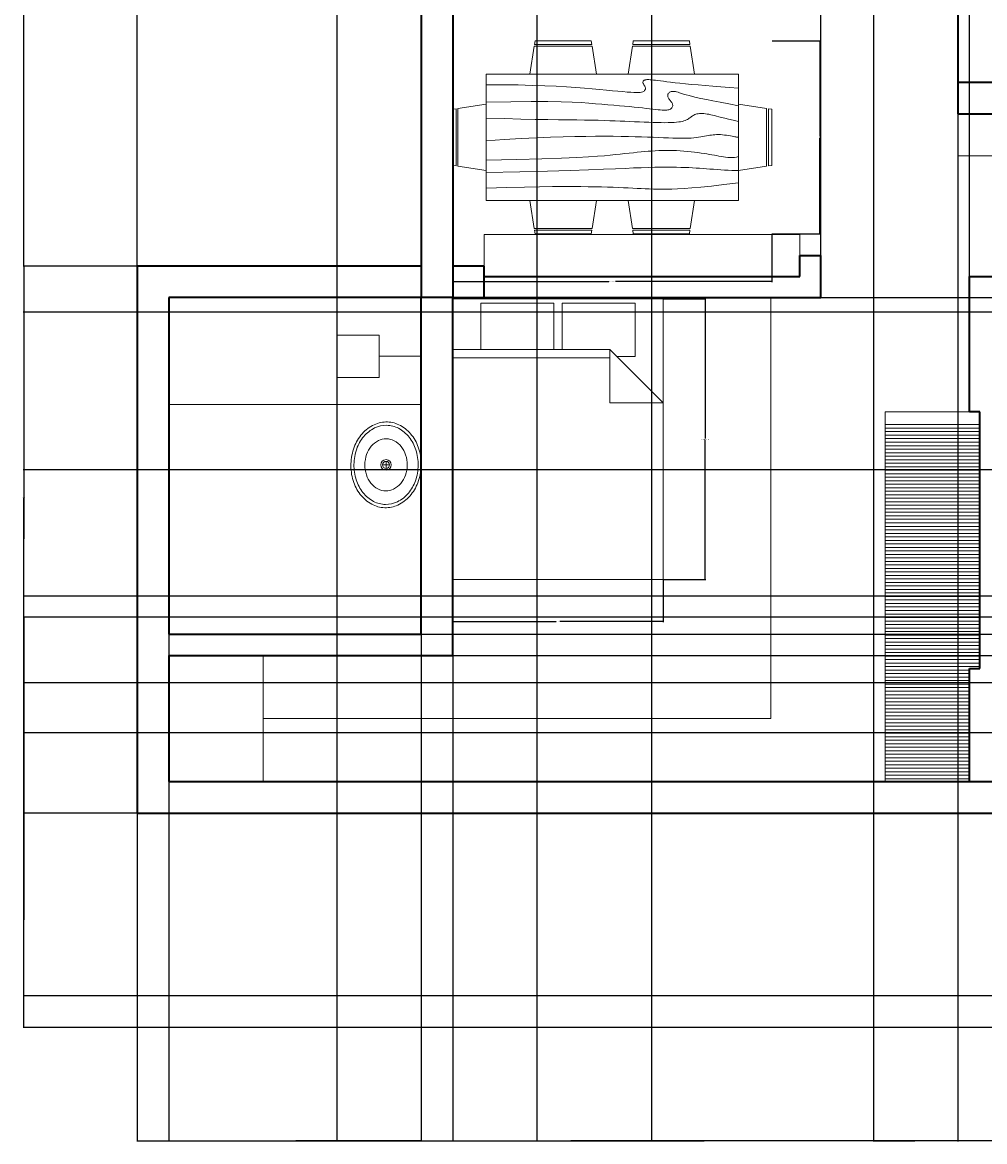
# Model space of a CAD drawing. Units: inches. Extents: x 1159 to 1869, y 2212 to 2738.
# Tile 1 of 5: x 1159 to 1433, y 2212 to 2531. Entities that reach past the tile are written whole.
import ezdxf

# ---------------------------------------------------------------- set-up
doc = ezdxf.new("R2010")
doc.units = ezdxf.units.IN
for name, color, linetype, lineweight in [('A-ANNO-DIMS', 2, 'Continuous', 18), ('A-FLOR', 9, 'Continuous', 13), ('A-FLOR-CASE', 30, 'Continuous', 18), ('A-FLOR-FIXT', 9, 'Continuous', 18), ('A-FLOR-PATT', 252, 'Continuous', 13), ('A-FURN', 8, 'Continuous', 18), ('A-WALL', 7, 'Continuous', 35)]:
    doc.layers.add(name, color=color, linetype=linetype, lineweight=lineweight)
doc.styles.get("Standard").update_dxf_attribs({"font": 'arial.ttf'})
doc.dimstyles.get("Standard").update_dxf_attribs({"dimtxt": 0.18, "dimasz": 0.18, "dimexe": 0.18, "dimexo": 0.0625, "dimgap": 0.09, "dimtad": 0, "dimtih": 1, "dimtoh": 1, "dimdec": 4, "dimzin": 0, "dimdsep": 46, "dimtxsty": 'Standard', "dimcen": 0.09, "dimadec": 0, "dimazin": 0, "dimtfac": 1, "dimtdec": 4, "dimtofl": 0, "dimtmove": 0, "dimatfit": 3, "dimfxl": 1, "dimtolj": 1, "dimtzin": 0, "dimarcsym": 0})

# ---------------------------------------------------------------- blocks, each defined once
blk = doc.blocks.new('Dining Set - 36 x 72 in.')
for p, q in [((-22.2343, 26.00059), (-23.4847, 17.99762)), ((-22.2304, 26), (-5.7608, 26)), ((-22, 27.5), (-22.1562, 26.50042)), ((-5.8416, 26.5), (-22.1534, 26.5)), ((-22, 27.5), (-6, 27.5)), ((-5.8437, 26.49966), (-6, 27.5)), ((-4.5152, 17.99762), (-5.7655, 25.99926)), ((5.7657, 26.00059), (4.5153, 17.99762)), ((5.7696, 26), (22.2392, 26)), ((6, 27.5), (5.8438, 26.50042)), ((22.1584, 26.5), (5.8466, 26.5)), ((6, 27.5), (22, 27.5)), ((22.1563, 26.49966), (22, 27.5)), ((23.4848, 17.99762), (22.2345, 25.99926)), ((36, 18), (-36, 18)), ((-36, 18), (-36, -18)), ((36, -18), (36, 18)), ((-45.5, 8), (-44.5004, 8.15617)), ((-45.5, 8), (-45.5, -8)), ((-44.5, -8.15843), (-44.5, 8.15338)), ((-44.0006, 8.23428), (-35.9976, 9.48474)), ((-44, 8.23041), (-44, -8.23915)), ((44.0006, 8.23428), (35.9976, 9.48474)), ((44, 8.23041), (44, -8.23915)), ((44.5, -8.15843), (44.5, 8.15338)), ((45.5, 8), (44.5005, 8.15617)), ((45.5, 8), (45.5, -8)), ((-44.4997, -8.15631), (-45.5, -8)), ((-35.9976, -9.48476), (-43.9993, -8.2345)), ((35.9976, -9.48476), (43.9993, -8.2345)), ((44.4997, -8.15631), (45.5, -8)), ((-36, -18), (36, -18)), ((-22.2343, -26.0006), (-23.4847, -17.99762)), ((-4.5152, -17.99762), (-5.7655, -25.99928)), ((5.7657, -26.0006), (4.5153, -17.99762)), ((23.4848, -17.99762), (22.2345, -25.99928)), ((-22.2304, -26), (-5.7608, -26)), ((-22, -27.5), (-22.1562, -26.50044)), ((-5.8416, -26.5), (-22.1534, -26.5)), ((-22, -27.5), (-6, -27.5)), ((-5.8437, -26.49967), (-6, -27.5)), ((5.7696, -26), (22.2392, -26)), ((6, -27.5), (5.8438, -26.50044)), ((22.1584, -26.5), (5.8466, -26.5)), ((6, -27.5), (22, -27.5)), ((22.1563, -26.49967), (22, -27.5))]:
    blk.add_line(p, q)
for points in [[(-36, 15), (-31.1772, 14.97754), (-26.8079, 14.91406), (-22.8538, 14.81543), (-19.276, 14.6875), (-16.0362, 14.53613), (-13.0957, 14.36718), (-10.4159, 14.18652), (-7.9583, 14), (-5.6904, 13.81315), (-3.6035, 13.63021), (-1.6954, 13.45508), (0.0365, 13.29166), (1.5945, 13.14388), (2.9811, 13.01562), (4.1988, 12.9108), (5.25, 12.83333), (6.1393, 12.78613), (6.8802, 12.76823), (7.4883, 12.77767), (7.9792, 12.8125), (8.3685, 12.87077), (8.6719, 12.95052), (8.9049, 13.0498), (9.0833, 13.16666), (9.2205, 13.29899), (9.3216, 13.44401), (9.3895, 13.59879), (9.4271, 13.76041), (9.4373, 13.92594), (9.4232, 14.09245), (9.3875, 14.257), (9.3333, 14.41666), (9.2638, 14.56917), (9.1836, 14.71484), (9.0975, 14.85465), (9.0104, 14.98958), (8.9272, 15.1206), (8.8529, 15.2487), (8.7922, 15.37483), (8.75, 15.5), (8.7305, 15.62467), (8.7344, 15.74739), (8.7617, 15.86621), (8.8125, 15.97916), (8.8867, 16.08431), (8.9844, 16.17968), (9.1055, 16.26334), (9.25, 16.33333), (9.4189, 16.38802), (9.6172, 16.42708), (9.8506, 16.45052), (10.125, 16.45833), (10.4463, 16.45052), (10.8203, 16.42708), (11.2529, 16.38802), (11.75, 16.33333), (12.3184, 16.26318), (12.9694, 16.17838), (13.7151, 16.07991), (14.5677, 15.96875), (15.5395, 15.84586), (16.6426, 15.71224), (17.8893, 15.56884), (19.2917, 15.41666), (20.859, 15.25667), (22.5879, 15.08984), (24.4721, 14.91715), (26.5052, 14.73958), (28.6809, 14.5581), (30.9929, 14.3737), (33.4347, 14.18733), (36, 14)], [(-36, 10), (-28.9766, 10.14274), (-23.1725, 10.20442), (-18.4241, 10.19775), (-14.5677, 10.13541), (-11.4399, 10.03011), (-8.877, 9.89453), (-6.7154, 9.74137), (-4.7917, 9.58333), (-2.9698, 9.43082), (-1.2246, 9.28515), (0.4415, 9.14534), (2.026, 9.01041), (3.5266, 8.87939), (4.9408, 8.7513), (6.266, 8.62516), (7.5, 8.5), (8.6411, 8.37549), (9.6914, 8.2539), (10.6538, 8.13818), (11.5312, 8.03125), (12.3267, 7.93603), (13.043, 7.85547), (13.6831, 7.79248), (14.25, 7.75), (14.7471, 7.7303), (15.1797, 7.73307), (15.5537, 7.75732), (15.875, 7.80208), (16.1494, 7.86637), (16.3828, 7.94922), (16.5811, 8.04964), (16.75, 8.16666), (16.8944, 8.29915), (17.0143, 8.44531), (17.1089, 8.60319), (17.1771, 8.77083), (17.218, 8.94629), (17.2305, 9.1276), (17.2137, 9.31282), (17.1667, 9.5), (17.0895, 9.6875), (16.987, 9.875), (16.8649, 10.0625), (16.7292, 10.25), (16.5856, 10.4375), (16.4401, 10.625), (16.2985, 10.8125), (16.1667, 11), (16.05, 11.18733), (15.9518, 11.3737), (15.8752, 11.5581), (15.8229, 11.73958), (15.798, 11.91715), (15.8034, 12.08984), (15.842, 12.25667), (15.9167, 12.41666), (16.0295, 12.56836), (16.1784, 12.70833), (16.3605, 12.83268), (16.5729, 12.9375), (16.8127, 13.01888), (17.0768, 13.07291), (17.3625, 13.0957), (17.6667, 13.08333), (17.9894, 13.03312), (18.3418, 12.94726), (18.7382, 12.82918), (19.1927, 12.68229), (19.7195, 12.51001), (20.3327, 12.31575), (21.0465, 12.10294), (21.875, 11.875), (22.8357, 11.63354), (23.959, 11.37304), (25.2786, 11.08618), (26.8282, 10.76562), (28.6414, 10.40405), (30.752, 9.99414), (33.1936, 9.52856), (36, 9)], [(-36, 5.5), (-30.7157, 5.3348), (-26.069, 5.20963), (-21.9946, 5.11767), (-18.4271, 5.05208), (-15.3009, 5.00602), (-12.5508, 4.97265), (-10.1112, 4.94515), (-7.9167, 4.91666), (-5.909, 4.88167), (-4.0586, 4.83984), (-2.3429, 4.79215), (-0.7396, 4.73958), (0.7739, 4.6831), (2.22, 4.6237), (3.6213, 4.56233), (5, 4.5), (6.373, 4.43782), (7.7344, 4.3776), (9.0723, 4.32129), (10.375, 4.27083), (11.6309, 4.22819), (12.8281, 4.19531), (13.9551, 4.17415), (15, 4.16666), (15.954, 4.17448), (16.819, 4.19791), (17.6001, 4.23698), (18.3021, 4.29166), (18.9299, 4.36198), (19.4883, 4.44791), (19.9823, 4.54948), (20.4167, 4.66666), (20.7969, 4.79899), (21.1302, 4.94401), (21.4245, 5.09879), (21.6875, 5.26041), (21.9271, 5.42594), (22.1511, 5.59245), (22.3672, 5.757), (22.5834, 5.91666), (22.8065, 6.06868), (23.0404, 6.21093), (23.2879, 6.34147), (23.5521, 6.45833), (23.8358, 6.55957), (24.142, 6.64323), (24.4735, 6.70735), (24.8334, 6.75), (25.2235, 6.76969), (25.642, 6.76692), (26.0858, 6.74267), (26.5521, 6.69791), (27.0379, 6.63362), (27.5404, 6.55078), (28.0565, 6.45036), (28.5834, 6.33333), (29.1242, 6.19987), (29.7071, 6.04687), (30.3661, 5.87044), (31.1354, 5.66666), (32.0493, 5.43164), (33.142, 5.16146), (34.4475, 4.85221), (36, 4.5)], [(-36, -1), (-30.7915, -0.6591), (-26.0195, -0.38216), (-21.6519, -0.16284), (-17.6563, 0.00521), (-14.0005, 0.12833), (-10.6523, 0.21289), (-7.5796, 0.26522), (-4.75, 0.29166), (-2.134, 0.29793), (0.2878, 0.28711), (2.5317, 0.26163), (4.6146, 0.22396), (6.5529, 0.17651), (8.3633, 0.12174), (10.0623, 0.06209), (11.6667, 0), (13.1899, -0.06201), (14.6341, -0.1211), (15.9982, -0.17432), (17.2813, -0.21875), (18.4823, -0.25147), (19.6003, -0.26953), (20.6343, -0.27002), (21.5834, -0.25), (22.4481, -0.20768), (23.2357, -0.14584), (23.9549, -0.06836), (24.6146, 0.02083), (25.2235, 0.11784), (25.7904, 0.21875), (26.3241, 0.31966), (26.8334, 0.41666), (27.3265, 0.50618), (27.8099, 0.58593), (28.2894, 0.65397), (28.7709, 0.70833), (29.2601, 0.74707), (29.763, 0.76823), (30.2855, 0.76985), (30.8334, 0.75), (31.4088, 0.70784), (31.9994, 0.64713), (32.589, 0.57275), (33.1615, 0.48958), (33.7008, 0.4025), (34.1908, 0.3164), (34.6153, 0.23616), (34.9584, 0.16666), (35.2099, 0.11165), (35.3848, 0.07031), (35.504, 0.04069), (35.5886, 0.02083), (35.6594, 0.00879), (35.7377, 0.0026), (35.8442, 0.00032), (36, 0)], [(-36, -6.5), (-27.1843, -6.31267), (-20.084, -6.1263), (-14.469, -5.9419), (-10.1094, -5.76042), (-6.7752, -5.58285), (-4.2363, -5.41016), (-2.2629, -5.24333), (-0.625, -5.08334), (0.8708, -4.93099), (2.2715, -4.78646), (3.5872, -4.64974), (4.8281, -4.52084), (6.0046, -4.39974), (7.127, -4.28646), (8.2053, -4.18099), (9.25, -4.08334), (10.2705, -3.99382), (11.2734, -3.91407), (12.2647, -3.84603), (13.25, -3.79167), (14.2354, -3.75293), (15.2266, -3.73177), (16.2295, -3.73015), (17.25, -3.75), (18.2912, -3.79248), (19.3451, -3.85547), (20.4009, -3.93604), (21.4479, -4.03125), (22.4754, -4.13819), (23.4727, -4.25391), (24.4289, -4.37549), (25.3334, -4.5), (26.1785, -4.62492), (26.9694, -4.74935), (27.7145, -4.87281), (28.4219, -4.99479), (29.1, -5.11483), (29.7572, -5.23242), (30.4016, -5.34709), (31.0417, -5.45834), (31.6837, -5.56437), (32.3262, -5.65821), (32.9658, -5.73153), (33.599, -5.77604), (34.2224, -5.78345), (34.8327, -5.74545), (35.4264, -5.65373), (36, -5.5)], [(-36, -10), (-26.4022, -9.81299), (-18.4675, -9.62891), (-11.9839, -9.45069), (-6.7396, -9.28125), (-2.5226, -9.12354), (0.8789, -8.98047), (3.6769, -8.85498), (6.0833, -8.75), (8.2767, -8.66765), (10.3021, -8.60677), (12.1712, -8.56543), (13.8958, -8.54167), (15.4876, -8.53353), (16.9583, -8.53907), (18.3197, -8.55632), (19.5834, -8.58334), (20.7616, -8.61841), (21.8685, -8.66081), (22.9188, -8.71004), (23.9271, -8.76563), (24.9081, -8.82707), (25.8763, -8.89388), (26.8465, -8.96558), (27.8334, -9.04167), (28.8474, -9.12118), (29.8828, -9.20117), (30.93, -9.27824), (31.9792, -9.34896), (33.0205, -9.40991), (34.0443, -9.45768), (35.0407, -9.48885), (36, -9.5)], [(-36, -14.5), (-30.0881, -14.33513), (-25.0332, -14.21224), (-20.7312, -14.12647), (-17.0781, -14.07292), (-13.97, -14.04671), (-11.3027, -14.04297), (-8.9724, -14.05681), (-6.875, -14.08334), (-4.9224, -14.11833), (-3.0905, -14.16016), (-1.3709, -14.20785), (0.2448, -14.26042), (1.7647, -14.3169), (3.1973, -14.3763), (4.5507, -14.43767), (5.8333, -14.5), (7.0554, -14.5621), (8.235, -14.62175), (9.3922, -14.67652), (10.5469, -14.72396), (11.7192, -14.76164), (12.929, -14.78711), (14.1965, -14.79794), (15.5417, -14.79167), (16.9933, -14.76424), (18.6152, -14.70508), (20.4804, -14.60197), (22.6615, -14.44271), (25.2312, -14.21509), (28.2624, -13.9069), (31.8277, -13.50594), (36, -13)]]:
    blk.add_lwpolyline(points)
blk = doc.blocks.new('Bed - Queen')
for p, q in [((0, -80.00003), (0, 0)), ((0, 0), (59.99999, 0)), ((59.99999, 0), (59.99999, -80.00003)), ((7.99999, -1.2), (28.79998, -1.2)), ((7.99999, -14.4), (7.99999, -1.2)), ((28.79998, -1.2), (28.79998, -14.4)), ((31.19999, -1.2), (51.99999, -1.2)), ((31.19999, -14.4), (31.19999, -1.2)), ((51.99999, -1.2), (51.99999, -16.4)), ((0, -14.4), (44.8, -14.4)), ((59.99999, -29.6), (44.8, -14.4)), ((44.8, -14.4), (44.8, -29.6)), ((44.8, -16.8), (0, -16.8)), ((51.99999, -16.4), (46.79936, -16.4)), ((44.8, -29.6), (59.99999, -29.6)), ((59.99999, -80.00003), (0, -80.00003))]:
    blk.add_line(p, q)
blk = doc.blocks.new('Sink - Oval top')
for p, q in [((-1, 0), (1, 0)), ((0, 1), (0, -1))]:
    blk.add_line(p, q)
for points in [[(-12.23, 0.39, 0.117634), (-11.46, -3.36, 0.104469), (-8.88, -6.8, 0.090016), (-5.08, -9.07, 0.08192), (-0.32, -10.02, 0.08192), (4.49, -9.38, 0.090016), (8.42, -7.36, 0.104469), (11.22, -4.09, 0.117634), (12.23, -0.39, 0.117634), (11.46, 3.36, 0.104469), (8.88, 6.8, 0.090016), (5.08, 9.07, 0.08192), (0.32, 10.02, 0.08192), (-4.49, 9.38, 0.090016), (-8.42, 7.36, 0.104469), (-11.22, 4.09, 0.117634)], [(-11.29, 0.16, 0.118622), (-10.52, -3.25, 0.104678), (-8.07, -6.36, 0.089562), (-4.54, -8.37, 0.081185), (-0.13, -9.15, 0.081185), (4.3, -8.49, 0.089562), (7.89, -6.58, 0.104678), (10.42, -3.55, 0.118622), (11.29, -0.16, 0.118622), (10.52, 3.25, 0.104678), (8.07, 6.36, 0.089562), (4.54, 8.37, 0.081185), (0.13, 9.15, 0.081185), (-4.3, 8.49, 0.089562), (-7.89, 6.58, 0.104678), (-10.42, 3.55, 0.118622)], [(-7.42, 0.08, 0.118283), (-6.91, -2.17, 0.104607), (-5.29, -4.21, 0.089718), (-2.97, -5.53, 0.081436), (-0.07, -6.04, 0.081436), (2.84, -5.59, 0.089718), (5.2, -4.33, 0.104607), (6.86, -2.32, 0.118283), (7.42, -0.08, 0.118283), (6.91, 2.17, 0.104607), (5.29, 4.21, 0.089718), (2.97, 5.53, 0.081436), (0.07, 6.04, 0.081436), (-2.84, 5.59, 0.089718), (-5.2, 4.33, 0.104607), (-6.86, 2.32, 0.118283)]]:
    blk.add_lwpolyline(points, format="xyb", close=True)
for radius in [1.5, 1]:
    blk.add_circle((0, 0), radius)
blk = doc.blocks.new('SHOWER-HEAD-SQUARE-12IN')
for p, q in [((6, 12), (0, 12)), ((0, 12), (0, 0)), ((12, 12), (6, 12)), ((12, 0), (12, 12)), ((0, 0), (12, 0))]:
    blk.add_line(p, q)
blk = doc.blocks.new('*D10')
at = {"layer": 'A-ANNO-DIMS', "color": 0, "lineweight": -2, "transparency": 16777216}
for p, q in [((1341.46, 2451.83), (1353.58, 2451.83)), ((1353.4, 2451.65), (1353.4, 2412.02)), ((1353.4, 2372.01), (1353.4, 2411.65)), ((1341.46, 2371.83), (1353.58, 2371.83))]:
    blk.add_line(p, q, dxfattribs=at)
at = {"layer": 'A-ANNO-DIMS', "color": 0, "transparency": 16777216}
for points in [[(1353.37, 2451.65), (1353.43, 2451.65), (1353.4, 2451.83)], [(1353.37, 2372.01), (1353.43, 2372.01), (1353.4, 2371.83)]]:
    blk.add_solid(points, dxfattribs=at)
at = {"layer": 'Defpoints', "color": 0, "transparency": 16777216}
for p in [(1341.4, 2451.83), (1353.4, 2451.83), (1341.4, 2371.83)]:
    blk.add_point(p, dxfattribs=at)
at = {"layer": 'A-ANNO-DIMS', "color": 0, "transparency": 16777216, "insert": (1353.4, 2411.83), "char_height": 0.18, "attachment_point": 5}
blk.add_mtext('\\A1;QUEEN BED 80 TYP.', dxfattribs=at)
blk = doc.blocks.new('*D11')
at = {"layer": 'A-ANNO-DIMS', "color": 0, "lineweight": -2, "transparency": 16777216}
for p, q in [((1281.4, 2371.77), (1281.4, 2359.65)), ((1341.4, 2371.77), (1341.4, 2359.65)), ((1281.58, 2359.83), (1310.87, 2359.83)), ((1341.22, 2359.83), (1311.93, 2359.83))]:
    blk.add_line(p, q, dxfattribs=at)
at = {"layer": 'A-ANNO-DIMS', "color": 0, "transparency": 16777216}
for points in [[(1281.58, 2359.86), (1281.58, 2359.8), (1281.4, 2359.83)], [(1341.22, 2359.86), (1341.22, 2359.8), (1341.4, 2359.83)]]:
    blk.add_solid(points, dxfattribs=at)
at = {"layer": 'Defpoints', "color": 0, "transparency": 16777216}
for p in [(1281.4, 2371.83), (1341.4, 2371.83), (1341.4, 2359.83)]:
    blk.add_point(p, dxfattribs=at)
at = {"layer": 'A-ANNO-DIMS', "color": 0, "transparency": 16777216, "insert": (1311.4, 2359.83), "char_height": 0.18, "attachment_point": 5}
blk.add_mtext('\\A1;60 TYP.', dxfattribs=at)
blk = doc.blocks.new('*D14')
at = {"layer": 'A-ANNO-DIMS', "color": 0, "lineweight": -2, "transparency": 16777216}
for p, q in [((1281.4, 2470.37), (1281.4, 2456.61)), ((1372.4, 2470.37), (1372.4, 2456.61)), ((1281.58, 2456.79), (1325.95, 2456.79)), ((1372.22, 2456.79), (1327.85, 2456.79))]:
    blk.add_line(p, q, dxfattribs=at)
at = {"layer": 'A-ANNO-DIMS', "color": 0, "transparency": 16777216}
for points in [[(1281.58, 2456.82), (1281.58, 2456.76), (1281.4, 2456.79)], [(1372.22, 2456.82), (1372.22, 2456.76), (1372.4, 2456.79)]]:
    blk.add_solid(points, dxfattribs=at)
at = {"layer": 'Defpoints', "color": 0, "transparency": 16777216}
for p in [(1281.4, 2470.44), (1372.4, 2470.44), (1372.4, 2456.79)]:
    blk.add_point(p, dxfattribs=at)
at = {"layer": 'A-ANNO-DIMS', "color": 0, "transparency": 16777216, "insert": (1326.9, 2456.79), "char_height": 0.18, "attachment_point": 5}
blk.add_mtext('\\A1;DINING SET 91', dxfattribs=at)
blk = doc.blocks.new('*D15')
at = {"layer": 'A-ANNO-DIMS', "color": 0, "lineweight": -2, "transparency": 16777216}
for p, q in [((1372.46, 2525.44), (1386.23, 2525.44)), ((1386.05, 2525.26), (1386.05, 2498.12)), ((1386.05, 2470.62), (1386.05, 2497.75)), ((1372.46, 2470.44), (1386.23, 2470.44))]:
    blk.add_line(p, q, dxfattribs=at)
at = {"layer": 'A-ANNO-DIMS', "color": 0, "transparency": 16777216}
for points in [[(1386.02, 2525.26), (1386.08, 2525.26), (1386.05, 2525.44)], [(1386.02, 2470.62), (1386.08, 2470.62), (1386.05, 2470.44)]]:
    blk.add_solid(points, dxfattribs=at)
at = {"layer": 'Defpoints', "color": 0, "transparency": 16777216}
for p in [(1372.4, 2525.44), (1386.05, 2525.44), (1372.4, 2470.44)]:
    blk.add_point(p, dxfattribs=at)
at = {"layer": 'A-ANNO-DIMS', "color": 0, "transparency": 16777216, "insert": (1386.05, 2497.94), "char_height": 0.18, "attachment_point": 5}
blk.add_mtext('\\A1;55', dxfattribs=at)
blk = doc.blocks.new('*D20')
at = {"layer": 'A-ANNO-DIMS', "color": 0, "lineweight": -2, "transparency": 16777216}
for p, q in [((1191.4, 2461.27), (1191.4, 2738.15)), ((1191.58, 2737.97), (1513.61, 2737.97)), ((1836.22, 2737.97), (1514.19, 2737.97)), ((1836.4, 2705.69), (1836.4, 2738.15))]:
    blk.add_line(p, q, dxfattribs=at)
at = {"layer": 'A-ANNO-DIMS', "color": 0, "transparency": 16777216}
for points in [[(1191.58, 2738), (1191.58, 2737.94), (1191.4, 2737.97)], [(1836.22, 2738), (1836.22, 2737.94), (1836.4, 2737.97)]]:
    blk.add_solid(points, dxfattribs=at)
at = {"layer": 'Defpoints', "color": 0, "transparency": 16777216}
for p in [(1836.4, 2737.97), (1836.4, 2705.63), (1191.4, 2461.21)]:
    blk.add_point(p, dxfattribs=at)
at = {"layer": 'A-ANNO-DIMS', "color": 0, "transparency": 16777216, "insert": (1513.9, 2737.97), "char_height": 0.18, "attachment_point": 5}
blk.add_mtext('\\A1;645', dxfattribs=at)
blk = doc.blocks.new('*D22')
at = {"layer": 'A-ANNO-DIMS', "color": 0, "lineweight": -2, "transparency": 16777216}
for p, q in [((1191.4, 2461.27), (1191.4, 2738.15)), ((1191.58, 2737.97), (1231.7, 2737.97)), ((1272.22, 2737.97), (1232.1, 2737.97)), ((1272.4, 2461.27), (1272.4, 2738.15))]:
    blk.add_line(p, q, dxfattribs=at)
at = {"layer": 'A-ANNO-DIMS', "color": 0, "transparency": 16777216}
for points in [[(1191.58, 2738), (1191.58, 2737.94), (1191.4, 2737.97)], [(1272.22, 2738), (1272.22, 2737.94), (1272.4, 2737.97)]]:
    blk.add_solid(points, dxfattribs=at)
at = {"layer": 'Defpoints', "color": 0, "transparency": 16777216}
for p in [(1272.4, 2737.97), (1191.4, 2461.21), (1272.4, 2461.21)]:
    blk.add_point(p, dxfattribs=at)
at = {"layer": 'A-ANNO-DIMS', "color": 0, "transparency": 16777216, "insert": (1231.9, 2737.97), "char_height": 0.18, "attachment_point": 5}
blk.add_mtext('\\A1;81', dxfattribs=at)
blk = doc.blocks.new('*D23')
at = {"layer": 'A-ANNO-DIMS', "color": 0, "lineweight": -2, "transparency": 16777216}
for p, q in [((1425.4, 2556.85), (1425.4, 2211.56)), ((1281.4, 2548.45), (1281.4, 2211.56)), ((1281.58, 2211.74), (1353.12, 2211.74)), ((1425.22, 2211.74), (1353.68, 2211.74))]:
    blk.add_line(p, q, dxfattribs=at)
at = {"layer": 'A-ANNO-DIMS', "color": 0, "transparency": 16777216}
for points in [[(1281.58, 2211.77), (1281.58, 2211.71), (1281.4, 2211.74)], [(1425.22, 2211.77), (1425.22, 2211.71), (1425.4, 2211.74)]]:
    blk.add_solid(points, dxfattribs=at)
at = {"layer": 'Defpoints', "color": 0, "transparency": 16777216}
for p in [(1425.4, 2556.91), (1281.4, 2548.52), (1425.4, 2211.74)]:
    blk.add_point(p, dxfattribs=at)
at = {"layer": 'A-ANNO-DIMS', "color": 0, "transparency": 16777216, "insert": (1353.4, 2211.74), "char_height": 0.18, "attachment_point": 5}
blk.add_mtext('\\A1;144', dxfattribs=at)
blk = doc.blocks.new('*D26')
at = {"layer": 'A-ANNO-DIMS', "color": 0, "lineweight": -2, "transparency": 16777216}
for p, q in [((1191.4, 2305.14), (1191.4, 2211.56)), ((1437.74, 2305.14), (1437.74, 2211.56)), ((1191.58, 2211.74), (1314.11, 2211.74)), ((1437.56, 2211.74), (1315.04, 2211.74))]:
    blk.add_line(p, q, dxfattribs=at)
at = {"layer": 'A-ANNO-DIMS', "color": 0, "transparency": 16777216}
for points in [[(1191.58, 2211.77), (1191.58, 2211.71), (1191.4, 2211.74)], [(1437.56, 2211.77), (1437.56, 2211.71), (1437.74, 2211.74)]]:
    blk.add_solid(points, dxfattribs=at)
at = {"layer": 'Defpoints', "color": 0, "transparency": 16777216}
for p in [(1191.4, 2305.21), (1437.74, 2305.21), (1437.74, 2211.74)]:
    blk.add_point(p, dxfattribs=at)
at = {"layer": 'A-ANNO-DIMS', "color": 0, "transparency": 16777216, "insert": (1314.57, 2211.74), "char_height": 0.18, "attachment_point": 5}
blk.add_mtext('\\A1;246.34', dxfattribs=at)
blk = doc.blocks.new('*D29')
at = {"layer": 'A-ANNO-DIMS', "color": 0, "lineweight": -2, "transparency": 16777216}
for p, q in [((1191.34, 2461.21), (1158.88, 2461.21)), ((1159.06, 2461.03), (1159.06, 2383.39)), ((1159.06, 2305.39), (1159.06, 2383.02)), ((1191.34, 2305.21), (1158.88, 2305.21))]:
    blk.add_line(p, q, dxfattribs=at)
at = {"layer": 'A-ANNO-DIMS', "color": 0, "transparency": 16777216}
for points in [[(1159.03, 2461.03), (1159.09, 2461.03), (1159.06, 2461.21)], [(1159.03, 2305.39), (1159.09, 2305.39), (1159.06, 2305.21)]]:
    blk.add_solid(points, dxfattribs=at)
at = {"layer": 'Defpoints', "color": 0, "transparency": 16777216}
for p in [(1159.06, 2461.21), (1191.4, 2461.21), (1191.4, 2305.21)]:
    blk.add_point(p, dxfattribs=at)
at = {"layer": 'A-ANNO-DIMS', "color": 0, "transparency": 16777216, "insert": (1159.06, 2383.21), "char_height": 0.18, "attachment_point": 5}
blk.add_mtext('\\A1;156', dxfattribs=at)
blk = doc.blocks.new('*D30')
at = {"layer": 'A-ANNO-DIMS', "color": 0, "lineweight": -2, "transparency": 16777216}
for p, q in [((1272.34, 2705.63), (1158.88, 2705.63)), ((1159.06, 2705.45), (1159.06, 2583.6)), ((1159.06, 2461.39), (1159.06, 2583.24)), ((1191.34, 2461.21), (1158.88, 2461.21))]:
    blk.add_line(p, q, dxfattribs=at)
at = {"layer": 'A-ANNO-DIMS', "color": 0, "transparency": 16777216}
for points in [[(1159.03, 2705.45), (1159.09, 2705.45), (1159.06, 2705.63)], [(1159.03, 2461.39), (1159.09, 2461.39), (1159.06, 2461.21)]]:
    blk.add_solid(points, dxfattribs=at)
at = {"layer": 'Defpoints', "color": 0, "transparency": 16777216}
for p in [(1159.06, 2705.63), (1272.4, 2705.63), (1191.4, 2461.21)]:
    blk.add_point(p, dxfattribs=at)
at = {"layer": 'A-ANNO-DIMS', "color": 0, "transparency": 16777216, "insert": (1159.06, 2583.42), "char_height": 0.18, "attachment_point": 5}
blk.add_mtext('\\A1;244.4', dxfattribs=at)
blk = doc.blocks.new('*D41')
at = {"layer": 'A-ANNO-DIMS', "color": 0, "lineweight": -2, "transparency": 16777216}
for p, q in [((1200.4, 2356.14), (1200.4, 2211.56)), ((1272.4, 2356.14), (1272.4, 2211.56)), ((1200.58, 2211.74), (1236.18, 2211.74)), ((1272.22, 2211.74), (1236.62, 2211.74))]:
    blk.add_line(p, q, dxfattribs=at)
at = {"layer": 'A-ANNO-DIMS', "color": 0, "transparency": 16777216}
for points in [[(1200.58, 2211.77), (1200.58, 2211.71), (1200.4, 2211.74)], [(1272.22, 2211.77), (1272.22, 2211.71), (1272.4, 2211.74)]]:
    blk.add_solid(points, dxfattribs=at)
at = {"layer": 'Defpoints', "color": 0, "transparency": 16777216}
for p in [(1200.4, 2356.21), (1272.4, 2356.21), (1272.4, 2211.74)]:
    blk.add_point(p, dxfattribs=at)
at = {"layer": 'A-ANNO-DIMS', "color": 0, "transparency": 16777216, "insert": (1236.4, 2211.74), "char_height": 0.18, "attachment_point": 5}
blk.add_mtext('\\A1;72', dxfattribs=at)
blk = doc.blocks.new('*D42')
at = {"layer": 'A-ANNO-DIMS', "color": 0, "lineweight": -2, "transparency": 16777216}
for p, q in [((1200.46, 2452.21), (1868.92, 2452.21)), ((1868.74, 2452.03), (1868.74, 2404.39)), ((1868.74, 2356.39), (1868.74, 2404.02)), ((1200.46, 2356.21), (1868.92, 2356.21))]:
    blk.add_line(p, q, dxfattribs=at)
at = {"layer": 'A-ANNO-DIMS', "color": 0, "transparency": 16777216}
for points in [[(1868.71, 2452.03), (1868.77, 2452.03), (1868.74, 2452.21)], [(1868.71, 2356.39), (1868.77, 2356.39), (1868.74, 2356.21)]]:
    blk.add_solid(points, dxfattribs=at)
at = {"layer": 'Defpoints', "color": 0, "transparency": 16777216}
for p in [(1200.4, 2452.21), (1868.74, 2452.21), (1200.4, 2356.21)]:
    blk.add_point(p, dxfattribs=at)
at = {"layer": 'A-ANNO-DIMS', "color": 0, "transparency": 16777216, "insert": (1868.74, 2404.21), "char_height": 0.18, "attachment_point": 5}
blk.add_mtext('\\A1;96', dxfattribs=at)
blk = doc.blocks.new('*D46')
at = {"layer": 'A-ANNO-DIMS', "color": 0, "lineweight": -2, "transparency": 16777216}
for p, q in [((1602.34, 2328.08), (1158.88, 2328.08)), ((1159.06, 2327.9), (1159.06, 2286.26)), ((1159.06, 2244.26), (1159.06, 2285.89)), ((1602.34, 2244.08), (1158.88, 2244.08))]:
    blk.add_line(p, q, dxfattribs=at)
at = {"layer": 'A-ANNO-DIMS', "color": 0, "transparency": 16777216}
for points in [[(1159.03, 2327.9), (1159.09, 2327.9), (1159.06, 2328.08)], [(1159.03, 2244.26), (1159.09, 2244.26), (1159.06, 2244.08)]]:
    blk.add_solid(points, dxfattribs=at)
at = {"layer": 'Defpoints', "color": 0, "transparency": 16777216}
for p in [(1159.06, 2328.08), (1602.4, 2328.08), (1602.4, 2244.08)]:
    blk.add_point(p, dxfattribs=at)
at = {"layer": 'A-ANNO-DIMS', "color": 0, "transparency": 16777216, "insert": (1159.06, 2286.08), "char_height": 0.18, "attachment_point": 5}
blk.add_mtext('\\A1;84', dxfattribs=at)
blk = doc.blocks.new('*D49')
at = {"layer": 'A-ANNO-DIMS', "color": 0, "lineweight": -2, "transparency": 16777216}
for p, q in [((1248.4, 2581.14), (1248.4, 2211.56)), ((1272.4, 2581.14), (1272.4, 2211.56)), ((1248.58, 2211.74), (1260.18, 2211.74)), ((1272.22, 2211.74), (1260.62, 2211.74))]:
    blk.add_line(p, q, dxfattribs=at)
at = {"layer": 'A-ANNO-DIMS', "color": 0, "transparency": 16777216}
for points in [[(1248.58, 2211.77), (1248.58, 2211.71), (1248.4, 2211.74)], [(1272.22, 2211.77), (1272.22, 2211.71), (1272.4, 2211.74)]]:
    blk.add_solid(points, dxfattribs=at)
at = {"layer": 'Defpoints', "color": 0, "transparency": 16777216}
for p in [(1248.4, 2581.21), (1272.4, 2581.21), (1272.4, 2211.74)]:
    blk.add_point(p, dxfattribs=at)
at = {"layer": 'A-ANNO-DIMS', "color": 0, "transparency": 16777216, "insert": (1260.4, 2211.74), "char_height": 0.18, "attachment_point": 5}
blk.add_mtext('\\A1;24', dxfattribs=at)
blk = doc.blocks.new('*D52')
at = {"layer": 'A-ANNO-DIMS', "color": 0, "lineweight": -2, "transparency": 16777216}
for p, q in [((1386.4, 2452.27), (1386.4, 2738.15)), ((1386.58, 2737.97), (1407.18, 2737.97)), ((1428.56, 2737.97), (1407.97, 2737.97)), ((1428.74, 2458.27), (1428.74, 2738.15))]:
    blk.add_line(p, q, dxfattribs=at)
at = {"layer": 'A-ANNO-DIMS', "color": 0, "transparency": 16777216}
for points in [[(1386.58, 2738), (1386.58, 2737.94), (1386.4, 2737.97)], [(1428.56, 2738), (1428.56, 2737.94), (1428.74, 2737.97)]]:
    blk.add_solid(points, dxfattribs=at)
at = {"layer": 'Defpoints', "color": 0, "transparency": 16777216}
for p in [(1428.74, 2737.97), (1428.74, 2458.21), (1386.4, 2452.21)]:
    blk.add_point(p, dxfattribs=at)
at = {"layer": 'A-ANNO-DIMS', "color": 0, "transparency": 16777216, "insert": (1407.57, 2737.97), "char_height": 0.18, "attachment_point": 5}
blk.add_mtext('\\A1;42.34', dxfattribs=at)
blk = doc.blocks.new('*D53')
at = {"layer": 'A-ANNO-DIMS', "color": 0, "lineweight": -2, "transparency": 16777216}
for p, q in [((1425.46, 2504.63), (1868.92, 2504.63)), ((1868.74, 2504.45), (1868.74, 2481.6)), ((1868.74, 2458.39), (1868.74, 2481.24)), ((1428.81, 2458.21), (1868.92, 2458.21))]:
    blk.add_line(p, q, dxfattribs=at)
at = {"layer": 'A-ANNO-DIMS', "color": 0, "transparency": 16777216}
for points in [[(1868.71, 2504.45), (1868.77, 2504.45), (1868.74, 2504.63)], [(1868.71, 2458.39), (1868.77, 2458.39), (1868.74, 2458.21)]]:
    blk.add_solid(points, dxfattribs=at)
at = {"layer": 'Defpoints', "color": 0, "transparency": 16777216}
for p in [(1425.4, 2504.63), (1868.74, 2504.63), (1428.74, 2458.21)]:
    blk.add_point(p, dxfattribs=at)
at = {"layer": 'A-ANNO-DIMS', "color": 0, "transparency": 16777216, "insert": (1868.74, 2481.42), "char_height": 0.18, "attachment_point": 5}
blk.add_mtext('\\A1;46.42', dxfattribs=at)
blk = doc.blocks.new('*D54')
at = {"layer": 'A-ANNO-DIMS', "color": 0, "lineweight": -2, "transparency": 16777216}
for p, q in [((1437.68, 2305.21), (1158.88, 2305.21)), ((1159.06, 2305.03), (1159.06, 2274.82)), ((1159.06, 2244.26), (1159.06, 2274.46)), ((1602.34, 2244.08), (1158.88, 2244.08))]:
    blk.add_line(p, q, dxfattribs=at)
at = {"layer": 'A-ANNO-DIMS', "color": 0, "transparency": 16777216}
for points in [[(1159.03, 2305.03), (1159.09, 2305.03), (1159.06, 2305.21)], [(1159.03, 2244.26), (1159.09, 2244.26), (1159.06, 2244.08)]]:
    blk.add_solid(points, dxfattribs=at)
at = {"layer": 'Defpoints', "color": 0, "transparency": 16777216}
for p in [(1437.74, 2305.21), (1159.06, 2244.08), (1602.4, 2244.08)]:
    blk.add_point(p, dxfattribs=at)
at = {"layer": 'A-ANNO-DIMS', "color": 0, "transparency": 16777216, "insert": (1159.06, 2274.64), "char_height": 0.18, "attachment_point": 5}
blk.add_mtext('\\A1;61.13', dxfattribs=at)
blk = doc.blocks.new('*D56')
at = {"layer": 'A-ANNO-DIMS', "color": 0, "lineweight": -2, "transparency": 16777216}
for p, q in [((1566.83, 2448.11), (1158.88, 2448.11)), ((1159.06, 2447.93), (1159.06, 2395.42)), ((1159.06, 2342.56), (1159.06, 2395.06)), ((1494.4, 2342.38), (1158.88, 2342.38))]:
    blk.add_line(p, q, dxfattribs=at)
at = {"layer": 'A-ANNO-DIMS', "color": 0, "transparency": 16777216}
for points in [[(1159.03, 2447.93), (1159.09, 2447.93), (1159.06, 2448.11)], [(1159.03, 2342.56), (1159.09, 2342.56), (1159.06, 2342.38)]]:
    blk.add_solid(points, dxfattribs=at)
at = {"layer": 'Defpoints', "color": 0, "transparency": 16777216}
for p in [(1566.9, 2448.11), (1159.06, 2342.38), (1494.46, 2342.38)]:
    blk.add_point(p, dxfattribs=at)
at = {"layer": 'A-ANNO-DIMS', "color": 0, "transparency": 16777216, "insert": (1159.06, 2395.24), "char_height": 0.18, "attachment_point": 5}
blk.add_mtext('\\A1;105.73', dxfattribs=at)
blk = doc.blocks.new('*D59')
at = {"layer": 'A-ANNO-DIMS', "color": 0, "lineweight": -2, "transparency": 16777216}
for p, q in [((1401.4, 2600.57), (1401.4, 2211.56)), ((1425.4, 2600.57), (1425.4, 2211.56)), ((1401.58, 2211.74), (1413.18, 2211.74)), ((1425.22, 2211.74), (1413.62, 2211.74))]:
    blk.add_line(p, q, dxfattribs=at)
at = {"layer": 'A-ANNO-DIMS', "color": 0, "transparency": 16777216}
for points in [[(1401.58, 2211.77), (1401.58, 2211.71), (1401.4, 2211.74)], [(1425.22, 2211.77), (1425.22, 2211.71), (1425.4, 2211.74)]]:
    blk.add_solid(points, dxfattribs=at)
at = {"layer": 'Defpoints', "color": 0, "transparency": 16777216}
for p in [(1401.4, 2600.63), (1425.4, 2600.63), (1425.4, 2211.74)]:
    blk.add_point(p, dxfattribs=at)
at = {"layer": 'A-ANNO-DIMS', "color": 0, "transparency": 16777216, "insert": (1413.4, 2211.74), "char_height": 0.18, "attachment_point": 5}
blk.add_mtext('\\A1;24', dxfattribs=at)
blk = doc.blocks.new('*D67')
at = {"layer": 'A-ANNO-DIMS', "color": 0, "lineweight": -2, "transparency": 16777216}
for p, q in [((1665.34, 2403.08), (1158.88, 2403.08)), ((1159.06, 2402.9), (1159.06, 2385.26)), ((1159.06, 2367.26), (1159.06, 2384.89)), ((1665.34, 2367.08), (1158.88, 2367.08))]:
    blk.add_line(p, q, dxfattribs=at)
at = {"layer": 'A-ANNO-DIMS', "color": 0, "transparency": 16777216}
for points in [[(1159.03, 2402.9), (1159.09, 2402.9), (1159.06, 2403.08)], [(1159.03, 2367.26), (1159.09, 2367.26), (1159.06, 2367.08)]]:
    blk.add_solid(points, dxfattribs=at)
at = {"layer": 'Defpoints', "color": 0, "transparency": 16777216}
for p in [(1159.06, 2403.08), (1665.4, 2403.08), (1665.4, 2367.08)]:
    blk.add_point(p, dxfattribs=at)
at = {"layer": 'A-ANNO-DIMS', "color": 0, "transparency": 16777216, "insert": (1159.06, 2385.08), "char_height": 0.18, "attachment_point": 5}
blk.add_mtext('\\A1;36', dxfattribs=at)
blk = doc.blocks.new('*D72')
at = {"layer": 'A-ANNO-DIMS', "color": 0, "lineweight": -2, "transparency": 16777216}
for p, q in [((1305.4, 2672.57), (1305.4, 2211.56)), ((1338.09, 2674.02), (1338.09, 2211.56)), ((1305.58, 2211.74), (1321.28, 2211.74)), ((1337.91, 2211.74), (1322.21, 2211.74))]:
    blk.add_line(p, q, dxfattribs=at)
at = {"layer": 'A-ANNO-DIMS', "color": 0, "transparency": 16777216}
for points in [[(1305.58, 2211.77), (1305.58, 2211.71), (1305.4, 2211.74)], [(1337.91, 2211.77), (1337.91, 2211.71), (1338.09, 2211.74)]]:
    blk.add_solid(points, dxfattribs=at)
at = {"layer": 'Defpoints', "color": 0, "transparency": 16777216}
for p in [(1305.4, 2672.63), (1338.09, 2674.08), (1338.09, 2211.74)]:
    blk.add_point(p, dxfattribs=at)
at = {"layer": 'A-ANNO-DIMS', "color": 0, "transparency": 16777216, "insert": (1321.74, 2211.74), "char_height": 0.18, "attachment_point": 5}
blk.add_mtext('\\A1;32.685', dxfattribs=at)
blk = doc.blocks.new('*D74')
at = {"layer": 'A-ANNO-DIMS', "color": 0, "lineweight": -2, "transparency": 16777216}
for p, q in [((1743.34, 2361.08), (1158.88, 2361.08)), ((1159.06, 2360.9), (1159.06, 2307.26)), ((1159.06, 2253.26), (1159.06, 2306.89)), ((1743.34, 2253.08), (1158.88, 2253.08))]:
    blk.add_line(p, q, dxfattribs=at)
at = {"layer": 'A-ANNO-DIMS', "color": 0, "transparency": 16777216}
for points in [[(1159.03, 2360.9), (1159.09, 2360.9), (1159.06, 2361.08)], [(1159.03, 2253.26), (1159.09, 2253.26), (1159.06, 2253.08)]]:
    blk.add_solid(points, dxfattribs=at)
at = {"layer": 'Defpoints', "color": 0, "transparency": 16777216}
for p in [(1159.06, 2361.08), (1743.4, 2361.08), (1743.4, 2253.08)]:
    blk.add_point(p, dxfattribs=at)
at = {"layer": 'A-ANNO-DIMS', "color": 0, "transparency": 16777216, "insert": (1159.06, 2307.08), "char_height": 0.18, "attachment_point": 5}
blk.add_mtext('\\A1;108', dxfattribs=at)
blk = doc.blocks.new('*D75')
at = {"layer": 'A-ANNO-DIMS', "color": 0, "lineweight": -2, "transparency": 16777216}
for p, q in [((1227.43, 2350.21), (1868.92, 2350.21)), ((1868.74, 2350.03), (1868.74, 2332.39)), ((1868.74, 2314.39), (1868.74, 2332.02)), ((1227.43, 2314.21), (1868.92, 2314.21))]:
    blk.add_line(p, q, dxfattribs=at)
at = {"layer": 'A-ANNO-DIMS', "color": 0, "transparency": 16777216}
for points in [[(1868.71, 2350.03), (1868.77, 2350.03), (1868.74, 2350.21)], [(1868.71, 2314.39), (1868.77, 2314.39), (1868.74, 2314.21)]]:
    blk.add_solid(points, dxfattribs=at)
at = {"layer": 'Defpoints', "color": 0, "transparency": 16777216}
for p in [(1227.37, 2350.21), (1868.74, 2350.21), (1227.37, 2314.21)]:
    blk.add_point(p, dxfattribs=at)
at = {"layer": 'A-ANNO-DIMS', "color": 0, "transparency": 16777216, "insert": (1868.74, 2332.21), "char_height": 0.18, "attachment_point": 5}
blk.add_mtext('\\A1;36', dxfattribs=at)

msp = doc.modelspace()

# ---------------------------------------------------------------- hatches: boundary and pattern name
at = {"layer": 'A-FLOR-PATT'}
h = msp.add_hatch(dxfattribs=at)
h.set_pattern_fill('ANSI31', color=256, scale=0.3149606, angle=-45, style=0)
h.paths.add_polyline_path([(1404.7443, 2314.8312), (1428.7443, 2314.8312), (1428.7443, 2346.4342), (1431.7443, 2346.4342), (1431.7443, 2416.8312), (1404.7443, 2416.8312)])

# ---------------------------------------------------------------- linework, layer by layer
at = {"layer": 'A-FLOR'}
for p, q in [((1372.067, 2452.2064), (1372.067, 2335.9511)), ((1227.3685, 2350.2064), (1227.3685, 2314.2064)), ((1372.067, 2332.2064), (1372.067, 2335.9511)), ((1227.3685, 2332.2064), (1372.067, 2332.2064))]:
    msp.add_line(p, q, dxfattribs=at)
at = {"layer": 'A-FLOR-CASE'}
for p, q in [((1425.4011, 2504.6279), (1425.4011, 2492.6279)), ((1425.4011, 2492.6279), (1549.9486, 2492.6279)), ((1380.4011, 2470.2064), (1290.4011, 2470.2064)), ((1290.4011, 2470.2064), (1290.4011, 2461.2064)), ((1380.4011, 2464.2064), (1380.4011, 2470.2064)), ((1404.7443, 2314.2064), (1404.7443, 2419.6143)), ((1428.7443, 2419.6143), (1404.7443, 2419.6143))]:
    msp.add_line(p, q, dxfattribs=at)
at = {"layer": 'A-FLOR-FIXT'}
for p, q in [((1272.4011, 2435.4781), (1260.4011, 2435.4781)), ((1272.4011, 2421.6999), (1200.4011, 2421.6999))]:
    msp.add_line(p, q, dxfattribs=at)
at = {"layer": 'A-WALL'}
for p, q in [((1425.4011, 2696.6279), (1425.4011, 2504.6279)), ((1272.4011, 2581.2064), (1272.4011, 2452.2064)), ((1281.4011, 2572.2064), (1281.4011, 2452.2064)), ((1425.4011, 2513.6279), (1569.4011, 2513.6279)), ((1425.4011, 2504.6279), (1443.4011, 2504.6279)), ((1380.4011, 2458.2064), (1380.4011, 2464.2064)), ((1380.4011, 2464.2064), (1386.4011, 2464.2064)), ((1386.4011, 2452.2064), (1386.4011, 2464.2064)), ((1191.4011, 2461.2064), (1191.4011, 2305.2064)), ((1272.4011, 2461.2064), (1191.4011, 2461.2064)), ((1290.4011, 2461.2064), (1281.4011, 2461.2064)), ((1290.4011, 2452.2064), (1290.4011, 2461.2064)), ((1290.4011, 2458.2064), (1380.4011, 2458.2064)), ((1428.7443, 2449.977), (1428.7443, 2458.2064)), ((1428.7443, 2458.2064), (1437.7443, 2458.2064)), ((1272.4011, 2452.2064), (1200.4011, 2452.2064)), ((1200.4011, 2452.2064), (1200.4011, 2356.2064)), ((1281.4011, 2452.2064), (1272.4011, 2452.2064)), ((1272.4011, 2356.2064), (1272.4011, 2452.2064)), ((1281.4011, 2350.2064), (1281.4011, 2452.2064)), ((1281.4011, 2452.2064), (1290.4011, 2452.2064)), ((1290.4011, 2452.2064), (1386.4011, 2452.2064)), ((1428.7443, 2419.6143), (1428.7443, 2449.977)), ((1431.7443, 2419.6143), (1428.7443, 2419.6143)), ((1431.7443, 2346.4342), (1431.7443, 2419.6143)), ((1200.4011, 2356.2064), (1272.4011, 2356.2064)), ((1200.4011, 2350.2064), (1281.4011, 2350.2064)), ((1200.4011, 2350.2064), (1200.4011, 2314.2064)), ((1428.7443, 2314.2064), (1428.7443, 2346.4342)), ((1428.7443, 2346.4342), (1431.7443, 2346.4342)), ((1200.4011, 2314.2064), (1437.7443, 2314.2064)), ((1191.4011, 2305.2064), (1437.7443, 2305.2064))]:
    msp.add_line(p, q, dxfattribs=at)

# ---------------------------------------------------------------- block references
at = {"layer": 'A-FLOR-FIXT'}
for name, p, rotation in [('SHOWER-HEAD-SQUARE-12IN', (1248.4014, 2441.4784), 269.9999999999998), ('Sink - Oval top', (1262.3853, 2404.5292), 90)]:
    msp.add_blockref(name, p, dxfattribs=dict(at, rotation=rotation))
at = {"layer": 'A-FURN'}
for name, p in [('Dining Set - 36 x 72 in.', (1326.9011, 2497.9351)), ('Bed - Queen', (1281.4011, 2451.8344))]:
    msp.add_blockref(name, p, dxfattribs=at)

# ---------------------------------------------------------------- dimensions: what is measured, and where the dimension line sits
at = {"layer": 'A-ANNO-DIMS'}
for base, p1, p2, override, picture, middle in [((1836.4011, 2737.9679), (1191.4011, 2461.2064), (1836.4011, 2705.6279), {"dimdec": 0, "dimlfac": 1, "dimrnd": 0, "dimzin": 0, "dimdsep": 46, "dimlunit": 2}, '*D20', (1513.9011, 2737.9679)), ((1272.4011, 2737.9679), (1191.4011, 2461.2064), (1272.4011, 2461.2064), {"dimdec": 0, "dimlfac": 1, "dimrnd": 0, "dimzin": 0, "dimdsep": 46, "dimlunit": 2}, '*D22', (1231.9011, 2737.9679)), ((1428.7443, 2737.9679), (1386.4011, 2452.2064), (1428.7443, 2458.2064), {"dimdec": 2, "dimlfac": 1, "dimrnd": 0, "dimzin": 0, "dimdsep": 46, "dimlunit": 2}, '*D52', (1407.5727, 2737.9679)), ((1338.0857, 2211.7357), (1305.4011, 2672.6279), (1338.0857, 2674.0796), {"dimdec": 3, "dimlfac": 1, "dimrnd": 0, "dimzin": 0, "dimdsep": 46, "dimlunit": 2}, '*D72', (1321.7434, 2211.7357)), ((1425.4011, 2211.7357), (1401.4011, 2600.6279), (1425.4011, 2600.6279), {"dimdec": 0, "dimlfac": 1, "dimrnd": 0, "dimzin": 0, "dimdsep": 46, "dimlunit": 2}, '*D59', (1413.4011, 2211.7357)), ((1272.4011, 2211.7357), (1248.4011, 2581.2064), (1272.4011, 2581.2064), {"dimdec": 0, "dimlfac": 1, "dimrnd": 0, "dimzin": 0, "dimdsep": 46, "dimlunit": 2}, '*D49', (1260.4011, 2211.7357)), ((1425.4011, 2211.7357), (1281.4011, 2548.5157), (1425.4011, 2556.9124), {"dimdec": 0, "dimlfac": 1, "dimrnd": 0, "dimzin": 0, "dimdsep": 46, "dimlunit": 2}, '*D23', (1353.4011, 2211.7357)), ((1272.4011, 2211.7357), (1200.4011, 2356.2064), (1272.4011, 2356.2064), {"dimdec": 0, "dimlfac": 1, "dimrnd": 0, "dimzin": 0, "dimdsep": 46, "dimlunit": 2}, '*D41', (1236.4011, 2211.7357)), ((1437.7443, 2211.7357), (1191.4011, 2305.2064), (1437.7443, 2305.2064), {"dimdec": 2, "dimlfac": 1, "dimrnd": 0, "dimzin": 0, "dimdsep": 46, "dimlunit": 2}, '*D26', (1314.5727, 2211.7357))]:
    dim = msp.add_linear_dim(base=base, p1=p1, p2=p2, dimstyle='Standard', override=override, dxfattribs=at)
    dim.commit()
    dim.dimension.update_dxf_attribs({"geometry": picture, "text_midpoint": middle})
for base, p1, p2, override, picture, middle in [((1159.0611, 2705.6279), (1191.4011, 2461.2064), (1272.4011, 2705.6279), {"dimdec": 1, "dimlfac": 1, "dimrnd": 0, "dimzin": 0, "dimdsep": 46, "dimlunit": 2}, '*D30', (1159.0611, 2583.4172)), ((1386.0511, 2525.4351), (1372.4011, 2470.4351), (1372.4011, 2525.4351), {"dimdec": 0, "dimlfac": 1, "dimrnd": 0, "dimzin": 0, "dimdsep": 46, "dimlunit": 2}, '*D15', (1386.0511, 2497.9351)), ((1868.7411, 2504.6279), (1428.7443, 2458.2064), (1425.4011, 2504.6279), {"dimdec": 2, "dimlfac": 1, "dimrnd": 0, "dimzin": 0, "dimdsep": 46, "dimlunit": 2}, '*D53', (1868.7411, 2481.4172)), ((1159.0611, 2461.2064), (1191.4011, 2305.2064), (1191.4011, 2461.2064), {"dimdec": 0, "dimlfac": 1, "dimrnd": 0, "dimzin": 0, "dimdsep": 46, "dimlunit": 2}, '*D29', (1159.0611, 2383.2064)), ((1868.7411, 2452.2064), (1200.4011, 2356.2064), (1200.4011, 2452.2064), {"dimdec": 0, "dimlfac": 1, "dimrnd": 0, "dimzin": 0, "dimdsep": 46, "dimlunit": 2}, '*D42', (1868.7411, 2404.2064)), ((1159.0611, 2342.3753), (1566.895, 2448.1096), (1494.4613, 2342.3753), {"dimdec": 2, "dimlfac": 1, "dimrnd": 0, "dimzin": 0, "dimdsep": 46, "dimlunit": 2}, '*D56', (1159.0611, 2395.2425)), ((1159.0611, 2403.0757), (1665.4011, 2367.0757), (1665.4011, 2403.0757), {"dimdec": 0, "dimlfac": 1, "dimrnd": 0, "dimzin": 0, "dimdsep": 46, "dimlunit": 2}, '*D67', (1159.0611, 2385.0757)), ((1159.0611, 2361.0757), (1743.4011, 2253.0757), (1743.4011, 2361.0757), {"dimdec": 0, "dimlfac": 1, "dimrnd": 0, "dimzin": 0, "dimdsep": 46, "dimlunit": 2}, '*D74', (1159.0611, 2307.0757)), ((1868.7411, 2350.2064), (1227.3685, 2314.2064), (1227.3685, 2350.2064), {"dimdec": 0, "dimlfac": 1, "dimrnd": 0, "dimzin": 0, "dimdsep": 46, "dimlunit": 2}, '*D75', (1868.7411, 2332.2064)), ((1159.0611, 2328.0757), (1602.4011, 2244.0757), (1602.4011, 2328.0757), {"dimdec": 0, "dimlfac": 1, "dimrnd": 0, "dimzin": 0, "dimdsep": 46, "dimlunit": 2}, '*D46', (1159.0611, 2286.0757)), ((1159.0611, 2244.0757), (1437.7443, 2305.2064), (1602.4011, 2244.0757), {"dimdec": 2, "dimlfac": 1, "dimrnd": 0, "dimzin": 0, "dimdsep": 46, "dimlunit": 2}, '*D54', (1159.0611, 2274.6411))]:
    dim = msp.add_linear_dim(base=base, p1=p1, p2=p2, angle=90, dimstyle='Standard', override=override, dxfattribs=at)
    dim.commit()
    dim.dimension.update_dxf_attribs({"geometry": picture, "text_midpoint": middle})
for base, p1, p2, text, picture, middle in [((1372.4011, 2456.7851), (1281.4011, 2470.4351), (1372.4011, 2470.4351), 'DINING SET <>', '*D14', (1326.9011, 2456.7851)), ((1341.4011, 2359.8344), (1281.4011, 2371.8344), (1341.4011, 2371.8344), '<> TYP.', '*D11', (1311.4011, 2359.8344))]:
    dim = msp.add_linear_dim(base=base, p1=p1, p2=p2, text=text, dimstyle='Standard', override={"dimdec": 0, "dimlfac": 1, "dimrnd": 0, "dimzin": 0, "dimdsep": 46, "dimlunit": 2}, dxfattribs=at)
    dim.commit()
    dim.dimension.update_dxf_attribs({"geometry": picture, "text_midpoint": middle})
dim = msp.add_linear_dim(base=(1353.4011, 2451.8344), p1=(1341.4011, 2371.8344), p2=(1341.4011, 2451.8344), angle=90, text='QUEEN BED <> TYP.', dimstyle='Standard', override={"dimdec": 0, "dimlfac": 1, "dimrnd": 0, "dimzin": 0, "dimdsep": 46, "dimlunit": 2}, dxfattribs=at)
dim.commit()
dim.dimension.update_dxf_attribs({"geometry": '*D10', "text_midpoint": (1353.4011, 2411.8344)})

doc.saveas('drawing.dxf')
